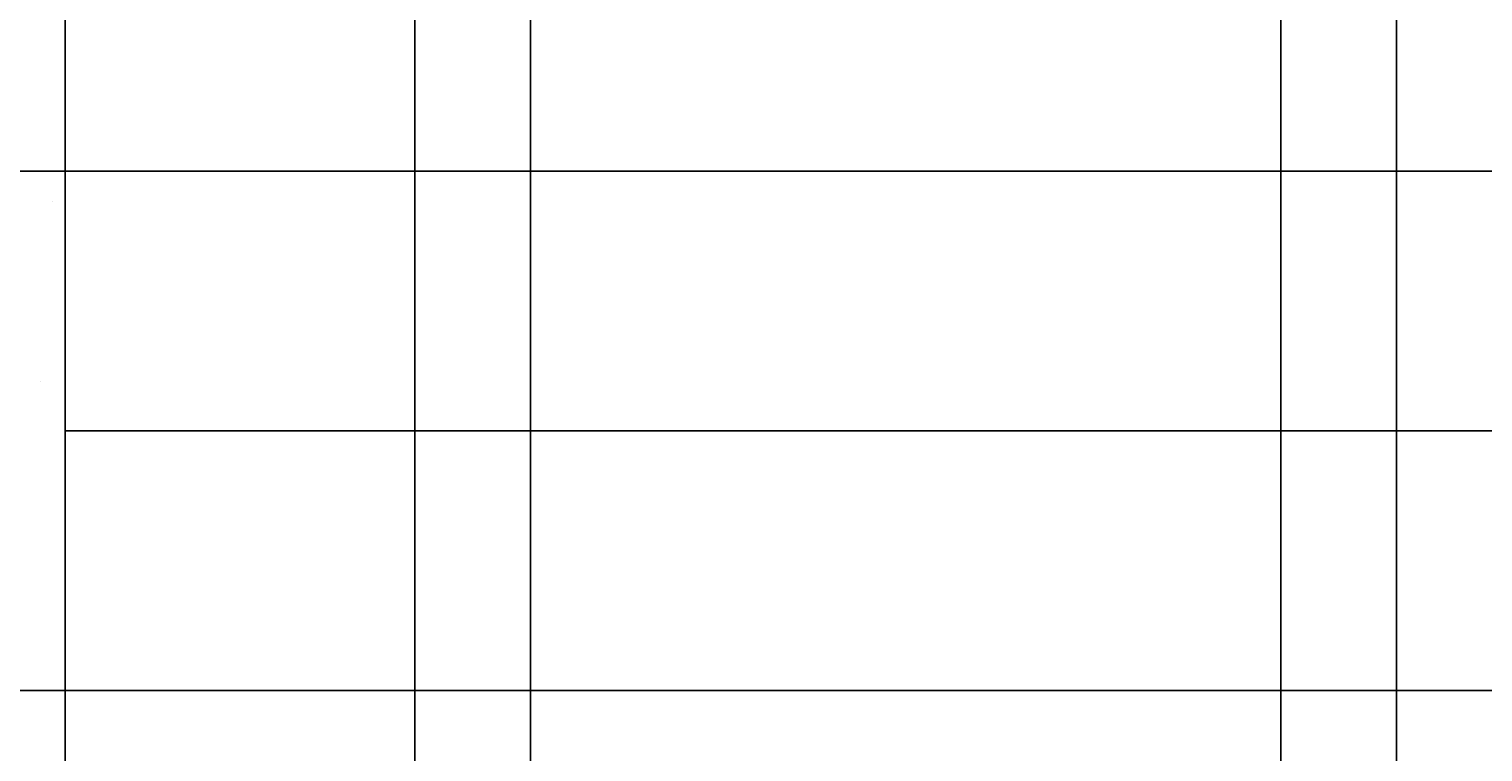
# Model space of a CAD drawing. Units: inches. Extents: x 37 to 824, y -700 to 234.
# Tile 11 of 77: x 298 to 348, y -606 to -581. Entities that reach past the tile are written whole.
import ezdxf

# ---------------------------------------------------------------- set-up
doc = ezdxf.new("R2010")
doc.units = ezdxf.units.IN
doc.header["$MEASUREMENT"] = 0
for name, color, linetype, lineweight in [('A-ANNO-DIMS', 2, 'Continuous', 18), ('A-ELEV', 3, 'Continuous', 25), ('A-ELEV-PATT', 8, 'Continuous', 13)]:
    doc.layers.add(name, color=color, linetype=linetype, lineweight=lineweight)
doc.styles.get("Standard").update_dxf_attribs({"font": 'arial.ttf'})
doc.dimstyles.get("Standard").update_dxf_attribs({"dimtxt": 0.18, "dimasz": 0.18, "dimexe": 0.18, "dimexo": 0.0625, "dimgap": 0.09, "dimtad": 0, "dimtih": 1, "dimtoh": 1, "dimdec": 1, "dimzin": 0, "dimdsep": 46, "dimlunit": 4, "dimtxsty": 'Standard', "dimcen": 0.09, "dimadec": 0, "dimazin": 0, "dimtfac": 1, "dimtdec": 1, "dimtofl": 0, "dimtmove": 0, "dimatfit": 3, "dimfxl": 1, "dimtolj": 1, "dimtzin": 0, "dimarcsym": 0})

# ---------------------------------------------------------------- blocks, each defined once
blk = doc.blocks.new('*D28')
at = {"layer": 'A-ANNO-DIMS', "color": 0, "lineweight": -2, "ltscale": 0.5, "transparency": 16777216}
for p, q in [((255.14, -537.627), (449.868, -537.627)), ((449.688, -543.627), (449.688, -558.537)), ((449.688, -579.627), (449.688, -564.717)), ((294.64, -585.627), (449.868, -585.627))]:
    blk.add_line(p, q, dxfattribs=at)
at = {"layer": 'A-ANNO-DIMS', "color": 0, "ltscale": 0.5, "transparency": 16777216}
for points in [[(448.688, -543.627), (450.688, -543.627), (449.688, -537.627)], [(448.688, -579.627), (450.688, -579.627), (449.688, -585.627)]]:
    blk.add_solid(points, dxfattribs=at)
at = {"layer": 'Defpoints', "color": 0, "ltscale": 0.5, "transparency": 16777216}
for p in [(255.077, -537.627), (294.577, -585.627), (449.688, -585.627)]:
    blk.add_point(p, dxfattribs=at)
at = {"layer": 'A-ANNO-DIMS', "color": 0, "ltscale": 0.5, "transparency": 16777216, "insert": (449.688, -561.627), "char_height": 6, "attachment_point": 5}
blk.add_mtext("\\A1;4'", dxfattribs=at)
blk = doc.blocks.new('*D69')
at = {"layer": 'A-ANNO-DIMS', "color": 0, "lineweight": -2, "ltscale": 0.5, "transparency": 16777216}
for p, q in [((255.077, -537.69), (255.077, -699.594)), ((299.077, -585.69), (299.077, -699.594)), ((255.257, -699.414), (276.748, -699.414)), ((298.897, -699.414), (277.406, -699.414))]:
    blk.add_line(p, q, dxfattribs=at)
at = {"layer": 'A-ANNO-DIMS', "color": 0, "ltscale": 0.5, "transparency": 16777216}
for points in [[(255.257, -699.384), (255.257, -699.444), (255.077, -699.414)], [(298.897, -699.384), (298.897, -699.444), (299.077, -699.414)]]:
    blk.add_solid(points, dxfattribs=at)
at = {"layer": 'Defpoints', "color": 0, "ltscale": 0.5, "transparency": 16777216}
for p in [(255.077, -537.627), (299.077, -585.627), (299.077, -699.414)]:
    blk.add_point(p, dxfattribs=at)
at = {"layer": 'A-ANNO-DIMS', "color": 0, "ltscale": 0.5, "transparency": 16777216, "insert": (277.077, -699.414), "char_height": 0.18, "attachment_point": 5}
blk.add_mtext('\\A1;3\'-8"', dxfattribs=at)
blk = doc.blocks.new('*D70')
at = {"layer": 'A-ANNO-DIMS', "color": 0, "lineweight": -2, "ltscale": 0.5, "transparency": 16777216}
for p, q in [((299.077, -585.69), (299.077, -699.594)), ((358.132, -585.69), (358.132, -699.594)), ((299.257, -699.414), (328.202, -699.414)), ((357.952, -699.414), (329.008, -699.414))]:
    blk.add_line(p, q, dxfattribs=at)
at = {"layer": 'A-ANNO-DIMS', "color": 0, "ltscale": 0.5, "transparency": 16777216}
for points in [[(299.257, -699.384), (299.257, -699.444), (299.077, -699.414)], [(357.952, -699.384), (357.952, -699.444), (358.132, -699.414)]]:
    blk.add_solid(points, dxfattribs=at)
at = {"layer": 'Defpoints', "color": 0, "ltscale": 0.5, "transparency": 16777216}
for p in [(299.077, -585.627), (358.132, -585.627), (358.132, -699.414)]:
    blk.add_point(p, dxfattribs=at)
at = {"layer": 'A-ANNO-DIMS', "color": 0, "ltscale": 0.5, "transparency": 16777216, "insert": (328.605, -699.414), "char_height": 0.18, "attachment_point": 5}
blk.add_mtext('\\A1;4\'-11"', dxfattribs=at)
blk = doc.blocks.new('*D102')
at = {"layer": 'A-ANNO-DIMS', "color": 0, "lineweight": -2, "ltscale": 0.5, "transparency": 16777216}
for p, q in [((311.196, -499.092), (311.196, -699.594)), ((345.196, -499.092), (345.196, -699.594)), ((311.376, -699.414), (327.795, -699.414)), ((345.016, -699.414), (328.596, -699.414))]:
    blk.add_line(p, q, dxfattribs=at)
at = {"layer": 'A-ANNO-DIMS', "color": 0, "ltscale": 0.5, "transparency": 16777216}
for points in [[(311.376, -699.384), (311.376, -699.444), (311.196, -699.414)], [(345.016, -699.384), (345.016, -699.444), (345.196, -699.414)]]:
    blk.add_solid(points, dxfattribs=at)
at = {"layer": 'Defpoints', "color": 0, "ltscale": 0.5, "transparency": 16777216}
for p in [(311.196, -499.03), (345.196, -499.03), (345.196, -699.414)]:
    blk.add_point(p, dxfattribs=at)
at = {"layer": 'A-ANNO-DIMS', "color": 0, "ltscale": 0.5, "transparency": 16777216, "insert": (328.196, -699.414), "char_height": 0.18, "attachment_point": 5}
blk.add_mtext('\\A1;2\'-10"', dxfattribs=at)
blk = doc.blocks.new('*D103')
at = {"layer": 'A-ANNO-DIMS', "color": 0, "lineweight": -2, "ltscale": 0.5, "transparency": 16777216}
for p, q in [((315.196, -505.092), (315.196, -699.594)), ((341.196, -505.092), (341.196, -699.594)), ((315.376, -699.414), (327.865, -699.414)), ((341.016, -699.414), (328.526, -699.414))]:
    blk.add_line(p, q, dxfattribs=at)
at = {"layer": 'A-ANNO-DIMS', "color": 0, "ltscale": 0.5, "transparency": 16777216}
for points in [[(315.376, -699.384), (315.376, -699.444), (315.196, -699.414)], [(341.016, -699.384), (341.016, -699.444), (341.196, -699.414)]]:
    blk.add_solid(points, dxfattribs=at)
at = {"layer": 'Defpoints', "color": 0, "ltscale": 0.5, "transparency": 16777216}
for p in [(315.196, -505.03), (341.196, -505.03), (341.196, -699.414)]:
    blk.add_point(p, dxfattribs=at)
at = {"layer": 'A-ANNO-DIMS', "color": 0, "ltscale": 0.5, "transparency": 16777216, "insert": (328.196, -699.414), "char_height": 0.18, "attachment_point": 5}
blk.add_mtext('\\A1;2\'-2"', dxfattribs=at)

msp = doc.modelspace()

# ---------------------------------------------------------------- hatches: boundary and pattern name
at = {"layer": 'A-ELEV-PATT', "ltscale": 0.5}
h = msp.add_hatch(dxfattribs=at)
h.set_pattern_fill('AR-BRSTD', color=256, scale=4)
h.paths.add_polyline_path([(299.077, -489.627), (358.132, -489.627), (358.132, -585.627), (428.077, -585.627), (428.077, -465.627), (161.077, -465.627), (161.077, -585.627), (299.077, -585.627)])
h.paths.add_polyline_path([(205.077, -537.627), (205.077, -489.627), (255.077, -489.627), (255.077, -537.627)], flags=16)
h = msp.add_hatch(dxfattribs=at)
h.set_pattern_fill('AR-CONC', color=256, scale=2)
h.paths.add_polyline_path([(299.077, -585.627), (161.077, -585.627), (161.077, -603.627), (299.077, -603.627)])
h.paths.add_polyline_path([(428.077, -585.627), (358.132, -585.627), (358.132, -603.627), (428.077, -603.627)])

# ---------------------------------------------------------------- linework, layer by layer
at = {"layer": 'A-ELEV', "ltscale": 0.5}
for p, q in [((299.077, -585.627), (358.132, -585.627)), ((299.077, -585.627), (299.077, -603.627)), ((299.077, -594.627), (358.132, -594.627))]:
    msp.add_line(p, q, dxfattribs=at)
for points in [[(161.077, -465.627), (428.077, -465.627), (428.077, -585.627), (161.077, -585.627)], [(299.077, -489.627), (358.132, -489.627), (358.132, -585.627), (299.077, -585.627)], [(161.077, -585.627), (428.077, -585.627), (428.077, -603.627), (161.077, -603.627)]]:
    msp.add_lwpolyline(points, close=True, dxfattribs=at)

# ---------------------------------------------------------------- dimensions: what is measured, and where the dimension line sits
at = {"layer": 'A-ANNO-DIMS', "ltscale": 0.5}
for base, p1, p2, picture, middle in [((345.196, -699.414), (311.196, -499.03), (345.196, -499.03), '*D102', (328.196, -699.414)), ((341.196, -699.414), (315.196, -505.03), (341.196, -505.03), '*D103', (328.196, -699.414)), ((299.077, -699.414), (255.077, -537.627), (299.077, -585.627), '*D69', (277.077, -699.414)), ((358.132, -699.414), (299.077, -585.627), (358.132, -585.627), '*D70', (328.605, -699.414))]:
    dim = msp.add_linear_dim(base=base, p1=p1, p2=p2, dimstyle='Standard', override={"dimdec": 1, "dimlfac": 1, "dimrnd": 0, "dimzin": 1, "dimdsep": 46, "dimlunit": 4, "dimfrac": 2}, dxfattribs=at)
    dim.commit()
    dim.dimension.update_dxf_attribs({"geometry": picture, "text_midpoint": middle})
dim = msp.add_linear_dim(base=(449.688, -585.627), p1=(255.077, -537.627), p2=(294.577, -585.627), angle=90, dimstyle='Standard', override={"dimtxt": 6, "dimasz": 6, "dimclrd": 0, "dimclre": 0, "dimclrt": 0}, dxfattribs=at)
dim.commit()
dim.dimension.update_dxf_attribs({"geometry": '*D28', "text_midpoint": (449.688, -561.627)})

doc.saveas('drawing.dxf')
